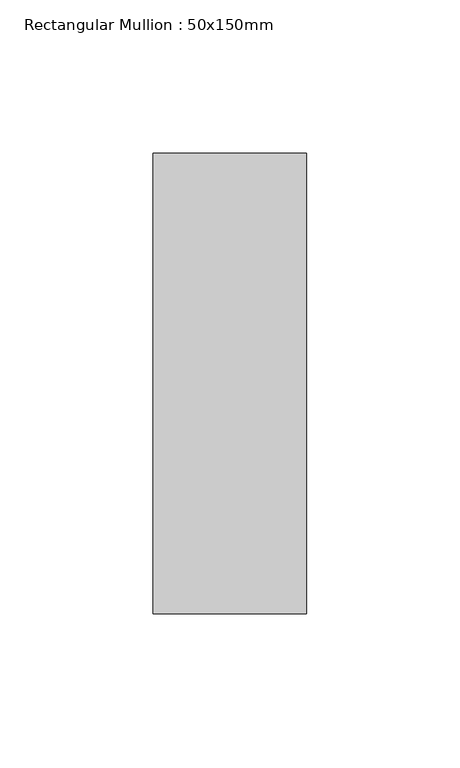
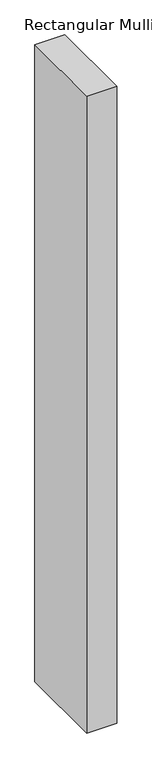
"""IFC4 building model written with IfcOpenShell, lengths in millimetres: member geometry, Rectangular Mullion : 50x150mm."""

from ifc_helpers import new_model, si_unit, frame, origin, place, context, project, spatial, polyline, outline, extrude, source, transform, mapped, element, save


def rectangular_mullion_50x150mm_60451361(model_context):
    return source(origin(), model_context, "Body", "SweptSolid", [
        extrude(outline(polyline([(0.0, 75.0), (0.0, -75.0), (-50.0, -75.0), (-50.0, 75.0), (0.0, 75.0)])), frame((0.0, 0.0, -1125.0), z_axis=(0.0, 0.0, 1.0), x_axis=(1.0, 0.0, 0.0)), (0.0, 0.0, 1.0), 1125.0),
    ])


if __name__ == "__main__":
    model = new_model("IFC4")
    model_context = context("Model", 3, world=origin())
    ifc_project = project(units=[si_unit("LENGTHUNIT", "METRE", prefix="MILLI")], contexts=[model_context])
    site = spatial("IfcSite", under=ifc_project)
    building = spatial("IfcBuilding", under=site)
    placement = place(None, origin())
    rectangular_mullion_50x150mm_shape = rectangular_mullion_50x150mm_60451361(model_context)
    element("IfcMember", 1, ObjectType="Rectangular Mullion : 50x150mm", at=placement, inside=building, context=model_context, shape_type="MappedRepresentation", body=[
        mapped(rectangular_mullion_50x150mm_shape, transform((0.0, 0.0, 0.0), x_axis=(1.0, 0.0, 0.0), y_axis=(0.0, 1.0, 0.0), z_axis=(0.0, 0.0, 1.0))),
    ])
    save(model, "model.ifc")

# Revit data of these elements
# Type "Rectangular Mullion : 50x150mm"
#   Keynote = "H11"
#   built-in parameter 1007304 = 0.492126 (stored number, unit not read)
#   built-in parameter 1007301 = 0.082021 (stored number, unit not read)
#   built-in parameter 1007300 = 0.082021 (stored number, unit not read)
# Element 1 (IfcMember, "Rectangular Mullion : 50x150mm")
#   Materials on its faces: "Aluminium"
# Materials
#   "Aluminium": class "Metal", colour RGB 247 247 247, transparency 0, Description = "Aluminium 6061", Cost = 0
